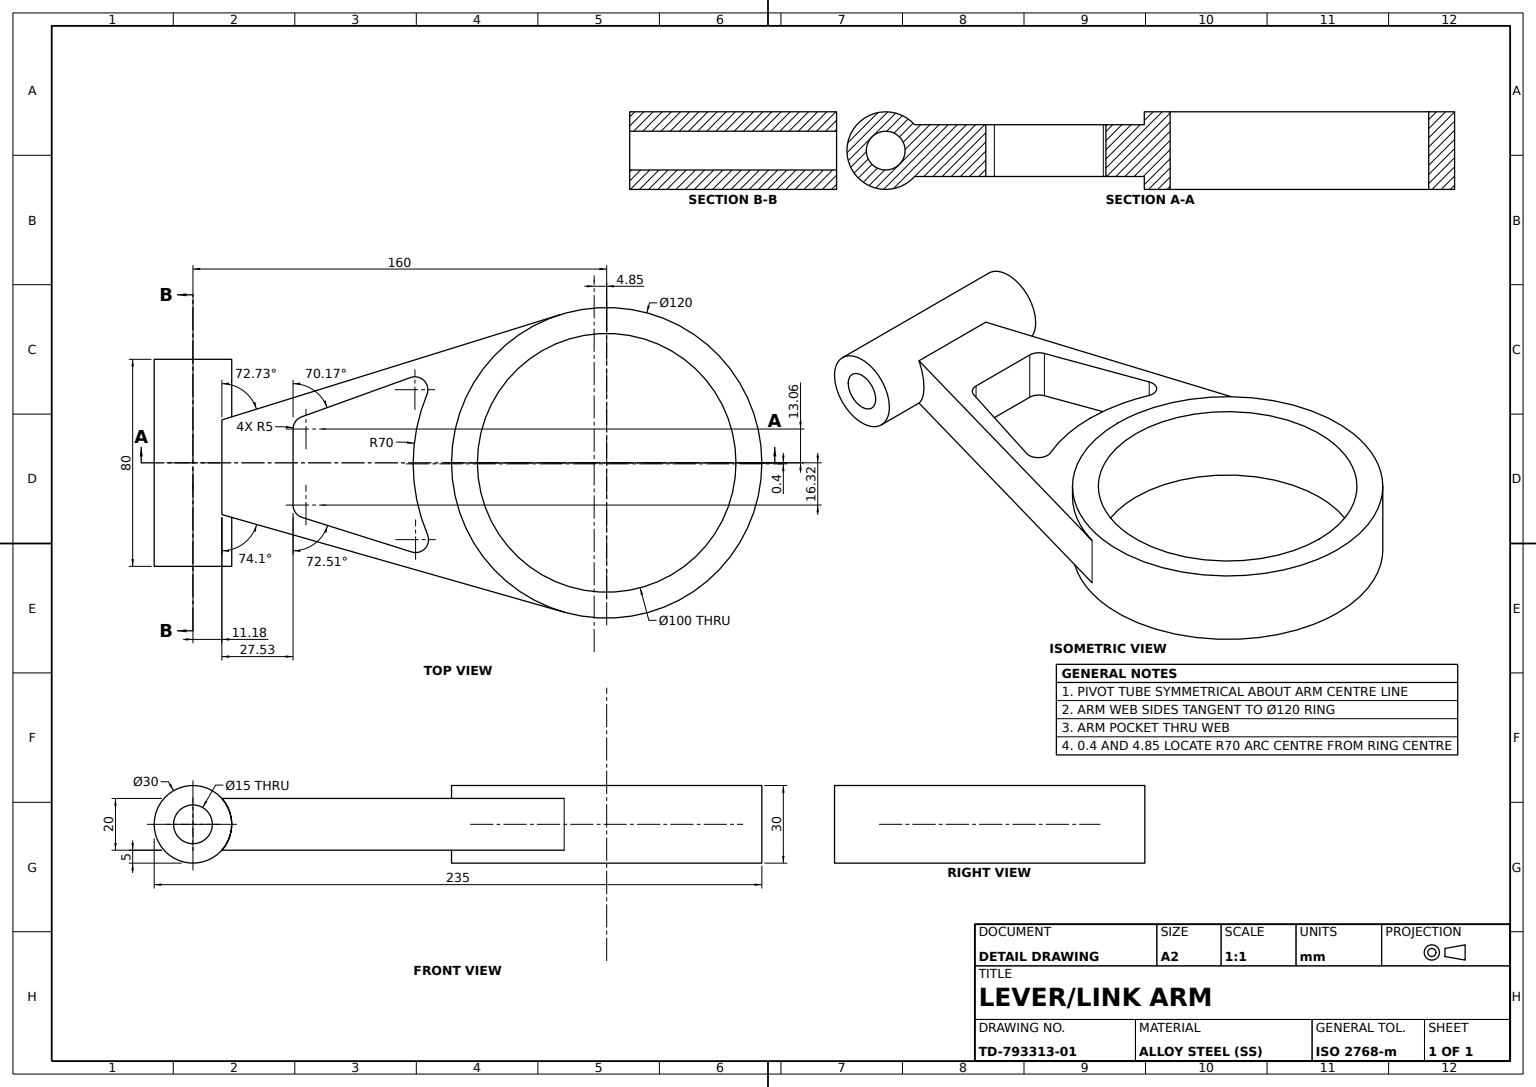
SolidWorks part; units mm, degrees
material "Alloy Steel (SS)"
ref_plane "Front Plane" through (0, 0, 0) normal (0, 0, 1) x (1, 0, 0)
ref_plane "Top Plane" through (0, 0, 0) normal (0, 1, 0) x (1, 0, 0)
ref_plane "Right Plane" through (0, 0, 0) normal (1, 0, 0) x (0, 0, -1)
sketch "Pivot Tube Sketch" plane through (0, 0, 0) normal (1, 0, 0) x (0, 0, -1)
  circle A0 centre (0, 0) radius 15
  circle A2 centre (0, 0) radius 7.5
  dimension "D1" = 15
  dimension "D2" = 30
extrude "Pivot Tube Ø30xØ15" add sketch "Pivot Tube Sketch" along normal mid plane 80
sketch "Arm Web Sketch" plane through (0, 0, 0) normal (0, 1, 0) x (1, 0, 0)
  line L0 (-16.4433, 10.7716) -> (19.8705, 10.7716)
  line L3 (-16.4433, 10.7716) -> (-57.2955, 142.1892)
  line L4 (19.8705, 10.7716) -> (57.7036, 143.5594)
  circle A0 centre (0, 160) radius 60
  circle A1 centre (0, 160) radius 50
  dimension "D1" = 100
  dimension "D2" = 120
  dimension "D3" = 160
  dimension "D4" = 36.3137
  dimension "D5" = 10.7716
  dimension "D6" = 16.4433
extrude "Arm Web 20mm" add sketch "Arm Web Sketch" along normal mid plane 20 contours A0 L3 L0 L4
sketch "Ring Hub Sketch" plane through (0, 0, 0) normal (0, 1, 0) x (1, 0, 0)
  line L0 (0, 0) -> (0, 160) construction
  circle A0 centre (0, 160) radius 50
  circle A1 centre (0, 160) radius 60
  dimension "D2" = 100
  dimension "D3" = 120
  dimension "D1" = 160
extrude "Ring Hub Ø120xØ100" add sketch "Ring Hub Sketch" along normal mid plane 30
sketch "Arm Pocket Sketch" plane through (0, 10, 0) normal (0, 1, 0) x (1, 0, 0)
  line L6 (-13.0584, 38.7136) -> (16.3202, 38.7136)
  line L7 (21.089, 42.2108) -> (34.4459, 84.5967)
  line L9 (-32.9546, 84.1411) -> (-17.7618, 42.0172)
  arc A2 (-26.3411, 90.4583) -> (27.7252, 90.7028) centre (0.4001, 155.1492) ccw
  arc A3 (-13.0584, 38.7136) -> (-17.7618, 42.0172) centre (-13.0584, 43.7136) cw
  arc A4 (16.3202, 38.7136) -> (21.089, 42.2108) centre (16.3202, 43.7136) ccw
  arc A5 (34.4459, 84.5967) -> (27.7252, 90.7028) centre (29.677, 86.0995) ccw
  arc A6 (-26.3411, 90.4583) -> (-32.9546, 84.1411) centre (-28.2512, 85.8375) ccw
  dimension "D1" = 70
  dimension "D2" = 5
  dimension "D3" = 23.2577
  dimension "D4" = 28.0266
  dimension "D5" = 29.9784
  dimension "D6" = 36.6146
  dimension "D7" = 70.762
  dimension "D8" = 75.4655
  dimension "D9" = 27.5333
extrude "Arm Lightening Pocket" cut sketch "Arm Pocket Sketch" against normal through all
